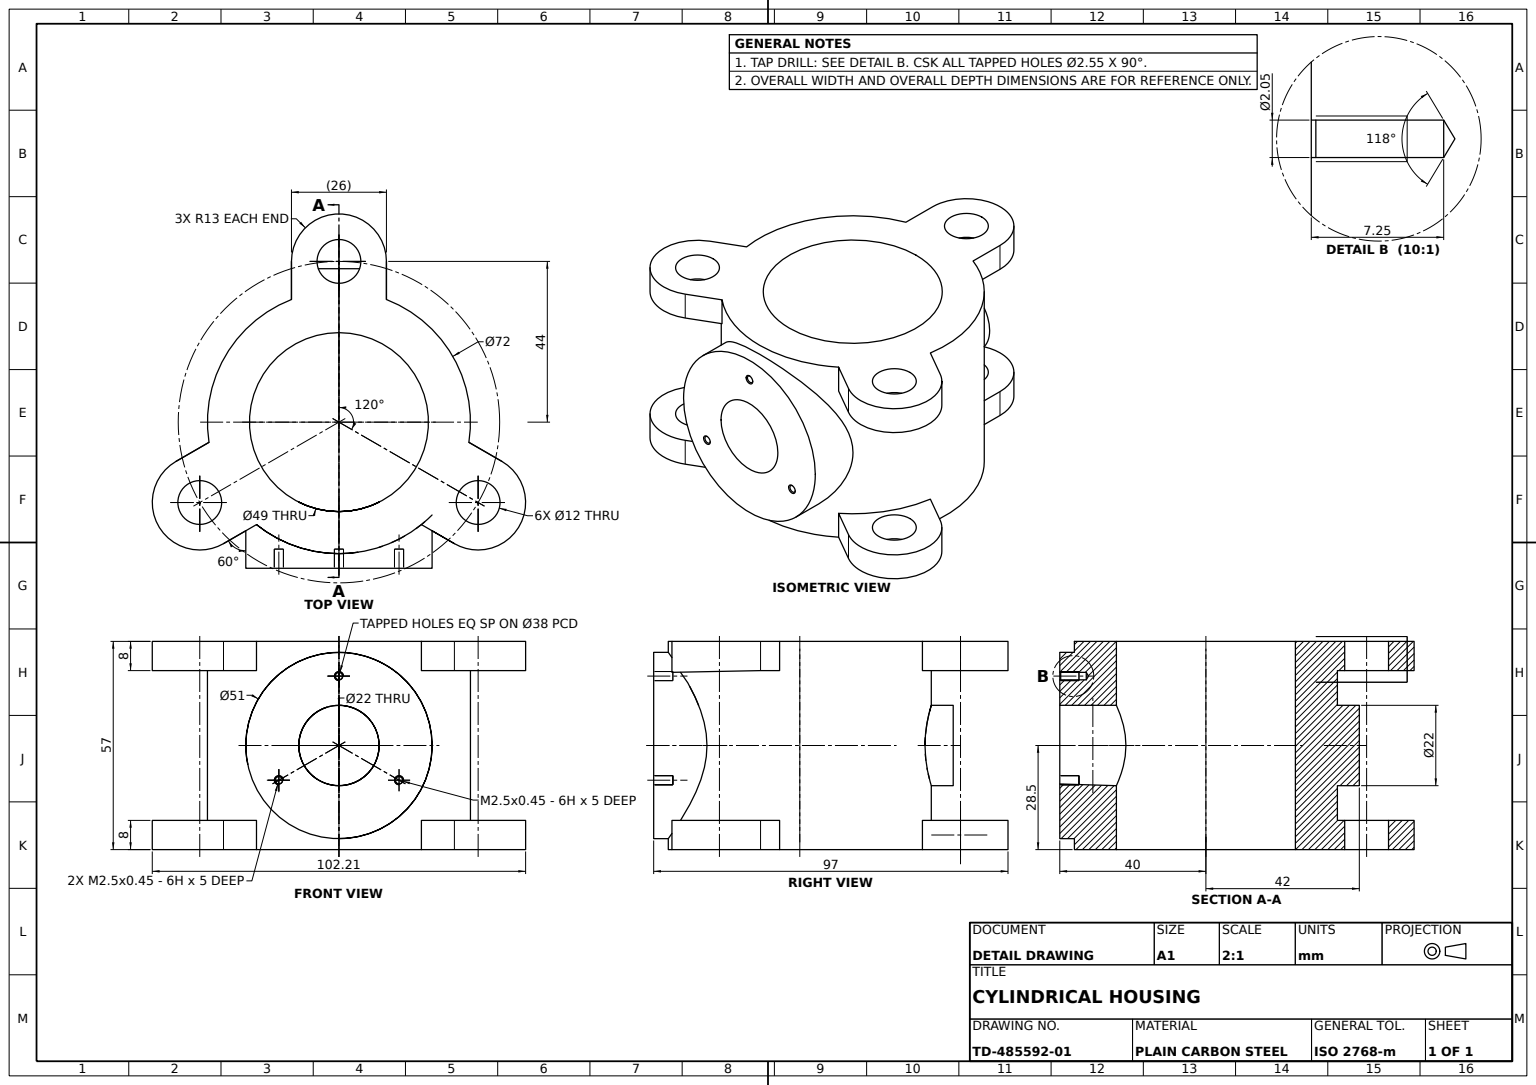
SolidWorks part; units mm, degrees
material "Plain Carbon Steel"
ref_plane "Front Plane" through (0, 0, 0) normal (0, 0, 1) x (1, 0, 0)
ref_plane "Top Plane" through (0, 0, 0) normal (0, 1, 0) x (1, 0, 0)
ref_plane "Right Plane" through (0, 0, 0) normal (1, 0, 0) x (0, 0, -1)
sketch "Main Body Profile Sketch" plane through (0, 0, 0) normal (0, 1, 0) x (1, 0, 0)
  circle A0 centre (0, 0) radius 36
  circle A1 centre (0, 0) radius 24.5
  dimension "D1" = 72
  dimension "D2" = 49
extrude "Main Body" add sketch "Main Body Profile Sketch" along normal mid plane 57
sketch "Mounting Lugs Sketch" plane through (0, 28.5, 0) normal (0, 1, 0) x (1, 0, 0)
  line L0 (-13, 44) -> (-13, 33.5708)
  line L1 (-13, 33.5708) -> (13, 33.5708)
  line L2 (13, 33.5708) -> (13, 44)
  line L3 (44.6051, -10.7417) -> (35.5732, -5.5271)
  line L4 (35.5732, -5.5271) -> (22.5732, -28.0437)
  line L5 (22.5732, -28.0437) -> (31.6051, -33.2583)
  line L6 (-31.6051, -33.2583) -> (-22.5732, -28.0437)
  line L7 (-22.5732, -28.0437) -> (-35.5732, -5.5271)
  line L8 (-35.5732, -5.5271) -> (-44.6051, -10.7417)
  arc A0 (13, 44) -> (-13, 44) centre (0, 44) ccw
  circle A1 centre (0, 0) radius 36 construction
  arc A2 (31.6051, -33.2583) -> (44.6051, -10.7417) centre (38.1051, -22) ccw
  arc A3 (-44.6051, -10.7417) -> (-31.6051, -33.2583) centre (-38.1051, -22) ccw
  circle A4 centre (0, 44) radius 6
  circle A5 centre (38.1051, -22) radius 6
  circle A6 centre (-38.1051, -22) radius 6
  dimension "D1" = 26
  dimension "D4" = 12
  dimension "D2" = 44
  dimension "D3" = 3
  dimension "D5" = 3
extrude "Top Mounting Lugs 3x" add sketch "Mounting Lugs Sketch" against normal blind 8
mirror "Bottom Mounting Lugs Mirror" about plane through (0, 0, 0) normal (0, 1, 0) of "Top Mounting Lugs 3x"
sketch "Side Port Boss Sketch Ø51" plane through (0, 0, 0) normal (0, 0, 1) x (1, 0, 0)
  circle A0 centre (0, 0) radius 25.5
  dimension "D1" = 51
extrude "Side Port Boss Ø51" add sketch "Side Port Boss Sketch Ø51" along normal blind 40
sketch "Port Tapped Hole Positions PCD38" plane through (0, 0, 40) normal (0, 0, 1) x (1, 0, 0)
  line L0 (0, 0) -> (0, 25.5) construction
  circle A0 centre (0, 0) radius 19 construction
  circle A1 centre (0, 0) radius 25.5 construction
  point P3 (0, 19)
  dimension "D1" = 38
hole_wizard "Port Tapped Hole M2.5" positions "3DSketch1" profile "Sketch5" tap size "M2.5x0.45" standard "ANSI Metric"
sketch3d "3DSketch1"
  point P0 (0, 19, 40)
sketch "Sketch5" plane through (0, 19, 40) normal (1, 0, 0) x (0, -1, 0)
  line L0 (0, 0) -> (0, 7.8659)
  line L1 (0, 7.8659) -> (1.025, 7.25)
  line L2 (1.025, 7.25) -> (1.025, 0.25)
  line L3 (1.025, 0.25) -> (1.275, 0)
  line L5 (1.275, 0) -> (0, 0)
  line L6 (-1.025, 0.25) -> (-1.275, 0) construction
  line L10 (0, 7.8659) -> (-1.025, 7.25) construction
  line L11 (0, -6.35) -> (0, 107.95) construction
  dimension "Tap Drill Dia." = 2.05
  dimension "Tap Drill Depth" = 7.25
  dimension "Near C'Sink Dia." = 2.55
  dimension "Near C'Sink Angle" = 90
  dimension "Drill Angle" = 118
cosmetic thread "Hole Thread1" parameters "D1"=5, "D2"=2.5
pattern_circular "Port Tapped Holes 3xM2.5 Pattern" count 3 over 360 about axis through (0, 0, 0) along (0, 0, 1) of "Port Tapped Hole M2.5"
cosmetic thread "Hole Thread2" parameters "D1"=5, "D2"=2.5
cosmetic thread "Hole Thread3" parameters "D1"=5, "D2"=2.5
sketch "Main Bore Sketch" plane through (0, 28.5, 0) normal (0, 1, 0) x (1, 0, 0)
  circle A0 centre (0, 0) radius 24.5 construction
  circle A1 centre (0, 0) radius 24.5
extrude "Main Bore" cut sketch "Main Bore Sketch" against normal through all
sketch "Side Port Bore Sketch Ø22" plane through (0, 0, 40) normal (0, 0, 1) x (1, 0, 0)
  circle A0 centre (0, 0) radius 11
  dimension "D1" = 22
extrude "Side Port Bore Ø22" cut sketch "Side Port Bore Sketch Ø22" against normal up to next
ref_plane "Internal Boss Plane" through (0, 0, -42) normal (0, 0, 1) x (1, 0, 0)
sketch "Internal Boss Sketch" plane through (0, 0, -42) normal (0, 0, 1) x (1, 0, 0)
  circle A0 centre (0, 0) radius 11 construction
  circle A1 centre (0, 0) radius 11
extrude "Internal Boss" add sketch "Internal Boss Sketch" along normal up to next
